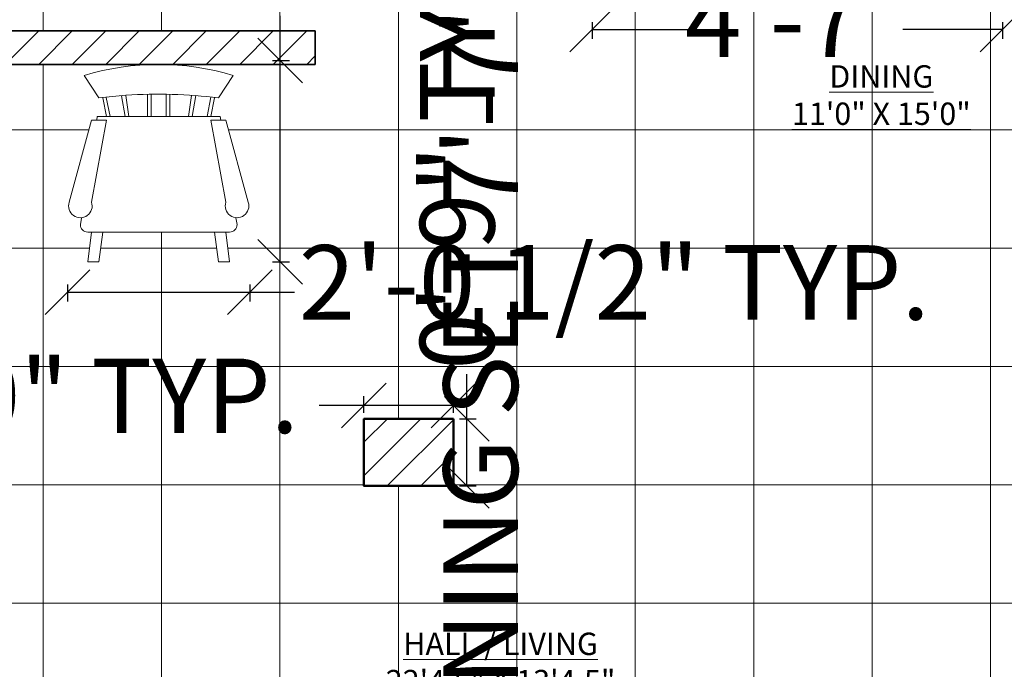
# Model space of a CAD drawing. Units: inches. Extents: x 2036 to 2670, y 319 to 920.
# Tile 5 of 15: x 2251 to 2383, y 579 to 666. Entities that reach past the tile are written whole.
import ezdxf

# ---------------------------------------------------------------- set-up
doc = ezdxf.new("R2010")
doc.units = ezdxf.units.IN
for name, color, linetype, lineweight in [('A-ANNO-DIMS', 2, 'Continuous', 18), ('A-AREA-IDEN', 7, 'Continuous', 18), ('A-COLS', 7, 'Continuous', 50), ('A-FLOR-PATT', 8, 'Continuous', 9), ('A-FURN', 8, 'Continuous', 18), ('A-WALL', 7, 'Continuous', 35)]:
    doc.layers.add(name, color=color, linetype=linetype, lineweight=lineweight)
doc.layers.add('A-COLS-PATT', color=240, linetype='Continuous', lineweight=13, true_color=0xed1f24)
doc.layers.add('A-WALL-PATT', color=52, linetype='Continuous', lineweight=13, true_color=0xc8c92d)
doc.styles.get("Standard").update_dxf_attribs({"font": 'arial.ttf'})
doc.dimstyles.new('ISO-25', dxfattribs={"dimtxt": 10, "dimasz": 6, "dimexe": 1.25, "dimexo": 0.625, "dimtad": 0, "dimdec": 1, "dimlunit": 3, "dimtxsty": 'Standard', "dimblk": 'OBLIQUE', "dimcen": 2.5, "dimclrd": 94, "dimclre": 94, "dimclrt": 1, "dimadec": 0, "dimazin": 0, "dimtfac": 1, "dimtdec": 1, "dimtmove": 0, "dimatfit": 3, "dimfxl": 1, "dimfxlon": 1, "dimarcsym": 0})

# ---------------------------------------------------------------- blocks, each defined once
blk = doc.blocks.new('Chair - Rocking')
for p, q in [((-8, -4.5), (-10, -1.5)), ((8, -4.5), (10, -1.5)), ((-7.5, -4.5), (-7, -7)), ((-6.5, -7), (-7.02225, -4.43)), ((-4.5, -7), (-4.96674, -4.19951)), ((-4, -7), (-4.40532, -4.16272)), ((-1.5, -4.05012), (-1.5, -7)), ((-1, -7), (-1, -4.05012)), ((1, -7), (1, -4.04655)), ((1.5, -4.05012), (1.5, -7)), ((4, -7), (4.40187, -4.18694)), ((4.5, -7), (4.96761, -4.19437)), ((6.5, -7), (7, -4.4057)), ((7.5, -4.5), (7, -7)), ((-9, -7.5), (-12, -18.49999)), ((-7, -7.5), (-9, -7.5)), ((-9, -18.49999), (-7, -7.5)), ((-8.23428, -6.99939), (-8.3093, -7.47958)), ((-8.23041, -7), (8.23915, -7)), ((7, -7.5), (9, -7.5)), ((9, -18.49999), (7, -7.5)), ((8.31071, -7.48854), (8.23449, -7.00073)), ((9, -7.5), (12, -18.49999)), ((-10.36644, -20.64523), (-10.5, -21.49999)), ((10.5, -21.49999), (10.3575, -20.58798)), ((-9, -22.49999), (-9.5, -26.49999)), ((0, -22.49999), (-9.5, -22.49999)), ((-8, -26.49999), (-7.5, -22.49999)), ((0, -22.49999), (9.5, -22.49999)), ((8, -26.49999), (7.5, -22.49999)), ((9, -22.49999), (9.5, -26.49999)), ((-9.5, -26.49999), (-8, -26.49999)), ((9.5, -26.49999), (8, -26.49999))]:
    blk.add_line(p, q)
for centre, radius, start, end in [((0, -34.08333), 34.08333, 72.93847, 107.0615), ((0, -68.25004), 64.25, 93.92211, 97.15267), ((0, -68.25004), 64.25, 82.84733, 93.92211), ((-10.5, -18.99999), 1.58114, 161.5651, 18.43495), ((10.5, -18.99999), 1.58114, 161.5651, 18.43495), ((-9.5, -21.49999), 1, 180, 270), ((9.5, -21.49999), 1, 270, 0)]:
    blk.add_arc(centre, radius, start, end)
blk = doc.blocks.new('COL-9x12')
blk.add_lwpolyline([(9, 0), (0, 0), (0, 12), (9, 12)], close=True)
blk = doc.blocks.new('_Oblique')
at = {"color": 0, "linetype": 'ByBlock', "lineweight": -2}
blk.add_line((-0.5, -0.5), (0.5, 0.5), dxfattribs=at)
blk = doc.blocks.new('*D21')
at = {"layer": 'A-ANNO-DIMS', "color": 94, "lineweight": -2, "transparency": 16777216}
for p, q in [((2297.27, 612.92), (2297.27, 615.17)), ((2309.27, 612.92), (2309.27, 615.17)), ((2297.27, 613.92), (2291.27, 613.92)), ((2309.27, 613.92), (2297.27, 613.92))]:
    blk.add_line(p, q, dxfattribs=at)
at = {"layer": 'Defpoints', "color": 0, "transparency": 16777216}
for p in [(2297.27, 613.92), (2297.27, 612.12), (2309.27, 612.12)]:
    blk.add_point(p, dxfattribs=at)
at = {"layer": 'A-ANNO-DIMS', "color": 94, "lineweight": -2, "transparency": 16777216, "xscale": 6, "yscale": 6, "zscale": 6}
for p, rotation in [((2297.27, 613.92), 179.9999999999962), ((2309.27, 613.92), 359.9999999999962)]:
    blk.add_blockref('_Oblique', p, dxfattribs=dict(at, rotation=rotation))
at = {"layer": 'A-ANNO-DIMS', "color": 1, "transparency": 16777216, "insert": (2228.01, 613.92), "char_height": 10, "attachment_point": 5}
blk.add_mtext('COLUMN 1\'-0" TYP.', dxfattribs=at)
blk = doc.blocks.new('*D22')
at = {"layer": 'A-ANNO-DIMS', "color": 94, "lineweight": -2, "transparency": 16777216}
for p, q in [((2311.07, 612.12), (2311.07, 618.12)), ((2310.07, 612.12), (2312.32, 612.12)), ((2311.07, 603.12), (2311.07, 612.12)), ((2310.07, 603.12), (2312.32, 603.12))]:
    blk.add_line(p, q, dxfattribs=at)
at = {"layer": 'Defpoints', "color": 0, "transparency": 16777216}
for p in [(2309.27, 612.12), (2311.07, 612.12), (2309.27, 603.12)]:
    blk.add_point(p, dxfattribs=at)
at = {"layer": 'A-ANNO-DIMS', "color": 94, "lineweight": -2, "transparency": 16777216, "xscale": 6, "yscale": 6, "zscale": 6}
for p, rotation in [((2311.07, 612.12), 90), ((2311.07, 603.12), 270)]:
    blk.add_blockref('_Oblique', p, dxfattribs=dict(at, rotation=rotation))
at = {"layer": 'A-ANNO-DIMS', "color": 1, "transparency": 16777216, "insert": (2311.07, 649.22), "char_height": 10, "attachment_point": 5, "rotation": 90}
blk.add_mtext('0\'-9" TYP.', dxfattribs=at)
blk = doc.blocks.new('*D23')
at = {"layer": 'A-ANNO-DIMS', "color": 94, "lineweight": -2, "transparency": 16777216}
for p, q in [((2286.03, 660.18), (2286.03, 666.18)), ((2285.03, 660.18), (2287.28, 660.18)), ((2286.03, 633.18), (2286.03, 660.18)), ((2285.03, 633.18), (2287.28, 633.18))]:
    blk.add_line(p, q, dxfattribs=at)
at = {"layer": 'Defpoints', "color": 0, "transparency": 16777216}
for p in [(2281.98, 660.18), (2286.03, 660.18), (2281.98, 633.18)]:
    blk.add_point(p, dxfattribs=at)
at = {"layer": 'A-ANNO-DIMS', "color": 94, "lineweight": -2, "transparency": 16777216, "xscale": 6, "yscale": 6, "zscale": 6}
for p, rotation in [((2286.03, 660.18), 90), ((2286.03, 633.18), 270)]:
    blk.add_blockref('_Oblique', p, dxfattribs=dict(at, rotation=rotation))
at = {"layer": 'A-ANNO-DIMS', "color": 1, "transparency": 16777216, "insert": (2286.03, 755.24), "char_height": 10, "attachment_point": 5, "rotation": 90}
blk.add_mtext('ROCKING CHAIR 2\'-3" TYP.', dxfattribs=at)
blk = doc.blocks.new('*D24')
at = {"layer": 'A-ANNO-DIMS', "color": 94, "lineweight": -2, "transparency": 16777216}
for p, q in [((2257.54, 630.13), (2257.54, 627.88)), ((2281.98, 630.13), (2281.98, 627.88)), ((2257.54, 629.13), (2281.98, 629.13)), ((2281.98, 629.13), (2287.98, 629.13))]:
    blk.add_line(p, q, dxfattribs=at)
at = {"layer": 'Defpoints', "color": 0, "transparency": 16777216}
for p in [(2257.54, 633.18), (2281.98, 633.18), (2281.98, 629.13)]:
    blk.add_point(p, dxfattribs=at)
at = {"layer": 'A-ANNO-DIMS', "color": 94, "lineweight": -2, "transparency": 16777216, "xscale": 6, "yscale": 6, "zscale": 6, "rotation": 180}
blk.add_blockref('_Oblique', (2257.54, 629.13), dxfattribs=at)
at = {"layer": 'A-ANNO-DIMS', "color": 94, "lineweight": -2, "transparency": 16777216, "xscale": 6, "yscale": 6, "zscale": 6}
blk.add_blockref('_Oblique', (2281.98, 629.13), dxfattribs=at)
at = {"layer": 'A-ANNO-DIMS', "color": 1, "transparency": 16777216, "insert": (2330.82, 629.13), "char_height": 10, "attachment_point": 5}
blk.add_mtext('2\'-0 1/2" TYP.', dxfattribs=at)
blk = doc.blocks.new('*D39')
at = {"layer": 'A-ANNO-DIMS', "color": 94, "lineweight": -2, "transparency": 16777216}
for p, q in [((2315.21, 769.01), (2312.96, 769.01)), ((2314.21, 769.01), (2314.21, 678.01)), ((2315.21, 678.01), (2312.96, 678.01)), ((2314.21, 678.01), (2314.21, 672.01))]:
    blk.add_line(p, q, dxfattribs=at)
at = {"layer": 'Defpoints', "color": 0, "transparency": 16777216}
for p in [(2327.86, 769.01), (2314.21, 678.01), (2327.86, 678.01)]:
    blk.add_point(p, dxfattribs=at)
at = {"layer": 'A-ANNO-DIMS', "color": 94, "lineweight": -2, "transparency": 16777216, "xscale": 6, "yscale": 6, "zscale": 6}
for p, rotation in [((2314.21, 769.01), 90), ((2314.21, 678.01), 270)]:
    blk.add_blockref('_Oblique', p, dxfattribs=dict(at, rotation=rotation))
at = {"layer": 'A-ANNO-DIMS', "color": 1, "transparency": 16777216, "insert": (2314.21, 616.43), "char_height": 10, "attachment_point": 5, "rotation": 90}
blk.add_mtext('DINING SET 7\'-7"', dxfattribs=at)
blk = doc.blocks.new('*D40')
at = {"layer": 'A-ANNO-DIMS', "color": 94, "lineweight": -2, "transparency": 16777216}
for p, q in [((2327.86, 665.36), (2327.86, 663.11)), ((2382.86, 665.36), (2382.86, 663.11)), ((2327.86, 664.36), (2341.24, 664.36)), ((2382.86, 664.36), (2369.48, 664.36))]:
    blk.add_line(p, q, dxfattribs=at)
at = {"layer": 'Defpoints', "color": 0, "transparency": 16777216}
for p in [(2327.86, 678.01), (2382.86, 678.01), (2382.86, 664.36)]:
    blk.add_point(p, dxfattribs=at)
at = {"layer": 'A-ANNO-DIMS', "color": 94, "lineweight": -2, "transparency": 16777216, "xscale": 6, "yscale": 6, "zscale": 6, "rotation": 180}
blk.add_blockref('_Oblique', (2327.86, 664.36), dxfattribs=at)
at = {"layer": 'A-ANNO-DIMS', "color": 94, "lineweight": -2, "transparency": 16777216, "xscale": 6, "yscale": 6, "zscale": 6}
blk.add_blockref('_Oblique', (2382.86, 664.36), dxfattribs=at)
at = {"layer": 'A-ANNO-DIMS', "color": 1, "transparency": 16777216, "insert": (2355.36, 664.36), "char_height": 10, "attachment_point": 5}
blk.add_mtext('4\'-7"', dxfattribs=at)
blk = doc.blocks.new('*D54')
at = {"layer": 'A-ANNO-DIMS', "color": 94, "lineweight": -2, "transparency": 16777216}
for p, q in [((2642.09, 545.51), (2642.09, 551.51)), ((2641.09, 545.51), (2643.34, 545.51)), ((2642.09, 513.19), (2642.09, 545.51)), ((2641.09, 513.19), (2643.34, 513.19))]:
    blk.add_line(p, q, dxfattribs=at)
at = {"layer": 'Defpoints', "color": 0, "transparency": 16777216}
for p in [(2158.74, 545.51), (2642.09, 545.51), (2158.74, 513.19)]:
    blk.add_point(p, dxfattribs=at)
at = {"layer": 'A-ANNO-DIMS', "color": 94, "lineweight": -2, "transparency": 16777216, "xscale": 6, "yscale": 6, "zscale": 6}
for p, rotation in [((2642.09, 545.51), 90), ((2642.09, 513.19), 270)]:
    blk.add_blockref('_Oblique', p, dxfattribs=dict(at, rotation=rotation))
at = {"layer": 'A-ANNO-DIMS', "color": 1, "transparency": 16777216, "insert": (2642.09, 577.16), "char_height": 10, "attachment_point": 5, "rotation": 90}
blk.add_mtext('2\'-8 1/2"', dxfattribs=at)
blk = doc.blocks.new('*D55')
at = {"layer": 'A-ANNO-DIMS', "color": 94, "lineweight": -2, "transparency": 16777216}
for p, q in [((2641.09, 582.53), (2643.34, 582.53)), ((2642.09, 582.53), (2642.09, 577.94)), ((2642.09, 545.51), (2642.09, 550.11)), ((2641.09, 545.51), (2643.34, 545.51))]:
    blk.add_line(p, q, dxfattribs=at)
at = {"layer": 'Defpoints', "color": 0, "transparency": 16777216}
for p in [(2158.74, 582.53), (2642.09, 582.53), (2158.74, 545.51)]:
    blk.add_point(p, dxfattribs=at)
at = {"layer": 'A-ANNO-DIMS', "color": 94, "lineweight": -2, "transparency": 16777216, "xscale": 6, "yscale": 6, "zscale": 6}
for p, rotation in [((2642.09, 582.53), 90), ((2642.09, 545.51), 270)]:
    blk.add_blockref('_Oblique', p, dxfattribs=dict(at, rotation=rotation))
at = {"layer": 'A-ANNO-DIMS', "color": 1, "transparency": 16777216, "insert": (2642.09, 564.02), "char_height": 10, "attachment_point": 5, "rotation": 90}
blk.add_mtext('3\'-1"', dxfattribs=at)
blk = doc.blocks.new('*D56')
at = {"layer": 'A-ANNO-DIMS', "color": 94, "lineweight": -2, "transparency": 16777216}
for p, q in [((2642.09, 599.85), (2642.09, 605.85)), ((2641.09, 599.85), (2643.34, 599.85)), ((2642.09, 582.53), (2642.09, 599.85)), ((2641.09, 582.53), (2643.34, 582.53))]:
    blk.add_line(p, q, dxfattribs=at)
at = {"layer": 'Defpoints', "color": 0, "transparency": 16777216}
for p in [(2158.74, 599.85), (2642.09, 599.85), (2158.74, 582.53)]:
    blk.add_point(p, dxfattribs=at)
at = {"layer": 'A-ANNO-DIMS', "color": 94, "lineweight": -2, "transparency": 16777216, "xscale": 6, "yscale": 6, "zscale": 6}
for p, rotation in [((2642.09, 599.85), 90), ((2642.09, 582.53), 270)]:
    blk.add_blockref('_Oblique', p, dxfattribs=dict(at, rotation=rotation))
at = {"layer": 'A-ANNO-DIMS', "color": 1, "transparency": 16777216, "insert": (2642.09, 630.95), "char_height": 10, "attachment_point": 5, "rotation": 90}
blk.add_mtext('1\'-5 1/2"', dxfattribs=at)
blk = doc.blocks.new('*D58')
at = {"layer": 'A-ANNO-DIMS', "color": 94, "lineweight": -2, "transparency": 16777216}
for p, q in [((2224.74, 436.33), (2224.74, 434.08)), ((2270.11, 436.33), (2270.11, 434.08)), ((2224.74, 435.33), (2270.11, 435.33)), ((2270.11, 435.33), (2276.11, 435.33))]:
    blk.add_line(p, q, dxfattribs=at)
at = {"layer": 'Defpoints', "color": 0, "transparency": 16777216}
for p in [(2224.74, 824.68), (2270.11, 824.68), (2270.11, 435.33)]:
    blk.add_point(p, dxfattribs=at)
at = {"layer": 'A-ANNO-DIMS', "color": 94, "lineweight": -2, "transparency": 16777216, "xscale": 6, "yscale": 6, "zscale": 6, "rotation": 180}
blk.add_blockref('_Oblique', (2224.74, 435.33), dxfattribs=at)
at = {"layer": 'A-ANNO-DIMS', "color": 94, "lineweight": -2, "transparency": 16777216, "xscale": 6, "yscale": 6, "zscale": 6}
blk.add_blockref('_Oblique', (2270.11, 435.33), dxfattribs=at)
at = {"layer": 'A-ANNO-DIMS', "color": 1, "transparency": 16777216, "insert": (2301.68, 435.33), "char_height": 10, "attachment_point": 5}
blk.add_mtext('3\'-9 1/2"', dxfattribs=at)
blk = doc.blocks.new('*D60')
at = {"layer": 'A-ANNO-DIMS', "color": 94, "lineweight": -2, "transparency": 16777216}
for p, q in [((2051.39, 582.41), (2051.39, 588.41)), ((2052.39, 582.41), (2050.14, 582.41)), ((2051.39, 545.09), (2051.39, 582.41)), ((2052.39, 545.09), (2050.14, 545.09))]:
    blk.add_line(p, q, dxfattribs=at)
at = {"layer": 'Defpoints', "color": 0, "transparency": 16777216}
for p in [(2051.39, 582.41), (2515.24, 582.41), (2515.24, 545.09)]:
    blk.add_point(p, dxfattribs=at)
at = {"layer": 'A-ANNO-DIMS', "color": 94, "lineweight": -2, "transparency": 16777216, "xscale": 6, "yscale": 6, "zscale": 6}
for p, rotation in [((2051.39, 582.41), 90), ((2051.39, 545.09), 270)]:
    blk.add_blockref('_Oblique', p, dxfattribs=dict(at, rotation=rotation))
at = {"layer": 'A-ANNO-DIMS', "color": 1, "transparency": 16777216, "insert": (2051.39, 613.98), "char_height": 10, "attachment_point": 5, "rotation": 90}
blk.add_mtext('3\'-1 1/2"', dxfattribs=at)

msp = doc.modelspace()

# ---------------------------------------------------------------- hatches: boundary and pattern name
at = {"layer": 'A-COLS-PATT'}
h = msp.add_hatch(dxfattribs=at)
h.set_pattern_fill('ANSI31', color=256)
h.paths.add_polyline_path([(2089.74, 875.68), (2080.74, 875.68), (2080.74, 863.68), (2089.74, 863.68)])
h.paths.add_polyline_path([(2089.74, 821.68), (2080.74, 821.68), (2080.74, 809.68), (2089.74, 809.68)])
h.paths.add_polyline_path([(2089.74, 624.2), (2080.74, 624.2), (2080.74, 612.2), (2089.74, 612.2)])
h.paths.add_polyline_path([(2158.74, 506.68), (2149.74, 506.68), (2149.74, 494.68), (2158.74, 494.68)])
h.paths.add_polyline_path([(2158.74, 617.33), (2149.74, 617.33), (2149.74, 605.33), (2158.74, 605.33)])
h.paths.add_polyline_path([(2158.74, 736.18), (2149.74, 736.18), (2149.74, 724.18), (2158.74, 724.18)])
h.paths.add_polyline_path([(2158.74, 852.81), (2149.74, 852.81), (2149.74, 843.81), (2158.74, 843.81)])
h.paths.add_polyline_path([(2161.74, 852.81), (2158.74, 852.81), (2158.74, 843.81), (2161.74, 843.81)])
h.paths.add_polyline_path([(2295.21, 857.66), (2290.74, 857.66), (2290.74, 848.68), (2295.21, 848.68)])
h.paths.add_polyline_path([(2290.74, 857.66), (2283.21, 857.66), (2283.21, 848.66), (2290.74, 848.66)])
h.paths.add_polyline_path([(2443.62, 857.68), (2431.62, 857.68), (2431.62, 848.68), (2443.62, 848.68)])
h.paths.add_polyline_path([(2561.81, 857.68), (2549.81, 857.68), (2549.81, 848.68), (2561.81, 848.68)])
h.paths.add_polyline_path([(2295.24, 737.65), (2290.74, 737.65), (2290.74, 728.68), (2295.24, 728.68)])
h.paths.add_polyline_path([(2309.27, 612.12), (2297.27, 612.12), (2297.27, 603.12), (2309.27, 603.12)])
h.paths.add_polyline_path([(2282.24, 503.68), (2270.24, 503.68), (2270.24, 494.68), (2282.24, 494.68)])
h.paths.add_polyline_path([(2431.74, 746.09), (2427.24, 746.09), (2427.24, 737.09), (2431.74, 737.09)])
h.paths.add_polyline_path([(2439.24, 746.09), (2431.74, 746.09), (2431.74, 737.09), (2439.24, 737.09)])
h.paths.add_polyline_path([(2596.59, 736.59), (2584.59, 736.59), (2584.59, 727.59), (2596.59, 727.59)])
h.paths.add_polyline_path([(2586.39, 623.71), (2574.39, 623.71), (2574.39, 619.18), (2586.39, 619.18)])
h.paths.add_polyline_path([(2586.39, 619.18), (2574.39, 619.18), (2574.39, 614.71), (2586.39, 614.71)])
h.paths.add_polyline_path([(2438.74, 623.68), (2431.24, 623.68), (2431.24, 619.18), (2438.74, 619.18)])
h.paths.add_polyline_path([(2438.74, 619.18), (2431.24, 619.18), (2431.24, 614.68), (2438.74, 614.68)])
h.paths.add_polyline_path([(2431.24, 623.68), (2426.74, 623.68), (2426.74, 614.68), (2431.24, 614.68), (2431.24, 619.18)])
h.paths.add_polyline_path([(2527.24, 503.68), (2515.24, 503.68), (2515.24, 494.68), (2527.24, 494.68)])
h.paths.add_polyline_path([(2590.31, 503.68), (2578.31, 503.68), (2578.31, 494.68), (2590.31, 494.68)])
at = {"layer": 'A-FLOR-PATT'}
h = msp.add_hatch(dxfattribs=at)
h.set_pattern_fill('ANSI31', color=256, scale=5, angle=135)
h.paths.add_polyline_path([(2290.74, 659.68), (2158.74, 659.68), (2158.74, 582.53), (2158.74, 545.51), (2158.74, 503.68), (2426.74, 503.68), (2426.74, 614.68), (2426.74, 623.68), (2426.74, 628.18), (2431.24, 628.18), (2431.24, 623.68), (2438.74, 623.68), (2438.74, 619.18), (2574.39, 619.18), (2574.39, 623.71), (2586.39, 623.71), (2586.39, 619.18), (2603.74, 619.18), (2603.74, 824.68), (2431.74, 824.68), (2431.74, 746.09), (2439.24, 746.09), (2439.24, 737.09), (2431.74, 737.09), (2431.74, 659.68), (2427.24, 659.68), (2427.24, 739.48), (2383.24, 739.48), (2383.24, 804.68), (2339.24, 804.68), (2339.24, 749.08), (2295.24, 749.08), (2295.24, 737.65), (2295.27, 737.65), (2295.27, 728.65), (2295.21, 728.65, -0.586418), (2272.74, 728.68), (2272.74, 824.68), (2270.11, 824.68), (2270.11, 829.18), (2290.74, 829.18), (2290.74, 848.66), (2283.21, 848.66), (2283.21, 857.66), (2289.74, 857.66), (2289.74, 874.68), (2158.74, 874.68), (2158.74, 852.81), (2161.74, 852.81), (2161.74, 843.81), (2158.74, 843.81), (2158.74, 829.18), (2224.74, 829.18), (2224.74, 800.68), (2182.74, 800.68), (2182.74, 733.41), (2158.74, 733.41), (2158.74, 728.68), (2235.24, 728.68), (2235.24, 714.81), (2230.74, 714.81), (2230.74, 724.18), (2158.74, 724.18), (2158.74, 664.18), (2230.74, 664.18), (2230.74, 678.81), (2235.24, 678.81), (2235.24, 664.18), (2290.74, 664.18)])
h.paths.add_polyline_path([(2309.27, 612.12), (2309.27, 603.12), (2297.27, 603.12), (2297.27, 612.12)], flags=16)
h.paths.add_polyline_path([(2280.12, 639.11), (2280.26, 638.18, -0.414214), (2279.26, 637.18), (2278.76, 637.18), (2279.26, 633.18), (2277.76, 633.18), (2277.26, 637.18), (2269.76, 637.18), (2262.26, 637.18), (2261.76, 633.18), (2260.26, 633.18), (2260.76, 637.18), (2260.26, 637.18, -0.414214), (2259.26, 638.18), (2259.41, 639.11, -0.541164), (2257.76, 641.18), (2260.76, 652.18), (2261.45, 652.18), (2261.53, 652.68), (2262.76, 652.68), (2262.25, 655.24, 0.001913), (2261.76, 655.18), (2259.76, 658.18, -0.15), (2279.76, 658.18), (2277.76, 655.18, 0.001913), (2277.27, 655.24), (2276.76, 652.68), (2278, 652.68), (2278.07, 652.18), (2278.76, 652.18), (2281.76, 641.18, -0.541163)], flags=16)
h.paths.add_polyline_path([(2245.98, 639.11), (2246.13, 638.18, -0.414214), (2245.13, 637.18), (2244.63, 637.18), (2245.13, 633.18), (2243.63, 633.18), (2243.13, 637.18), (2235.63, 637.18), (2228.13, 637.18), (2227.63, 633.18), (2226.13, 633.18), (2226.63, 637.18), (2226.13, 637.18, -0.414214), (2225.13, 638.18), (2225.27, 639.11, -0.541164), (2223.63, 641.18), (2226.63, 652.18), (2227.32, 652.18), (2227.39, 652.68), (2228.63, 652.68), (2228.12, 655.24, 0.001913), (2227.63, 655.18), (2225.63, 658.18, -0.15), (2245.63, 658.18), (2243.63, 655.18, 0.001913), (2243.14, 655.24), (2242.63, 652.68), (2243.86, 652.68), (2243.94, 652.18), (2244.63, 652.18), (2247.63, 641.18, -0.541163)], flags=16)
h.paths.add_polyline_path([(2351.59, 515.15, -0.151948), (2279.59, 515.15), (2279.59, 537.68), (2273.59, 537.68), (2273.59, 511.68, 0.190476), (2357.59, 511.68), (2357.59, 537.68), (2351.59, 537.68)])
h.paths.add_polyline_path([(2327.59, 536.13), (2327.59, 517.07), (2303.59, 517.07), (2303.59, 536.13)], flags=16)
h.paths.add_polyline_path([(2213.4, 639.11), (2213.55, 638.18, -0.414214), (2212.55, 637.18), (2212.05, 637.18), (2212.55, 633.18), (2211.05, 633.18), (2210.55, 637.18), (2203.05, 637.18), (2195.55, 637.18), (2195.05, 633.18), (2193.55, 633.18), (2194.05, 637.18), (2193.55, 637.18, -0.414214), (2192.55, 638.18), (2192.69, 639.11, -0.541164), (2191.05, 641.18), (2194.05, 652.18), (2194.73, 652.18), (2194.81, 652.68), (2196.05, 652.68), (2195.53, 655.24, 0.001913), (2195.05, 655.18), (2193.05, 658.18, -0.15), (2213.05, 658.18), (2211.05, 655.18, 0.001913), (2210.56, 655.24), (2210.05, 652.68), (2211.28, 652.68), (2211.36, 652.18), (2212.05, 652.18), (2215.05, 641.18, -0.541163)], flags=16)
h.paths.add_polyline_path([(2368.58, 538.02), (2370.52, 538.02), (2371.17, 532.84), (2380.89, 532.84), (2390.6, 532.84), (2391.25, 538.02), (2393.2, 538.02), (2392.55, 532.84), (2380.89, 532.84), (2368.58, 532.84, 0.414214), (2367.28, 531.54), (2367.47, 530.34, -0.483352), (2369.23, 527.65), (2371.82, 513.4), (2370.12, 513.4), (2370.22, 512.75), (2391.56, 512.75), (2391.66, 513.4), (2389.96, 513.4), (2392.55, 527.65, -1.387427), (2396.43, 527.65), (2392.55, 513.4), (2391.66, 513.4), (2391.56, 512.75), (2389.31, 512.75), (2390, 509.37, 0.003796), (2391.25, 509.51), (2393.84, 505.63, -0.15), (2367.93, 505.63), (2370.52, 509.51, 0.003901), (2371.81, 509.36), (2372.47, 512.75), (2370.22, 512.75), (2370.12, 513.4), (2369.23, 513.4), (2365.34, 527.65, -0.541163), (2367.47, 530.34), (2367.28, 531.54, -0.414214), (2368.58, 532.84), (2369.23, 532.84)])
h.paths.add_polyline_path([(2266.74, 538.02), (2266.09, 532.84), (2254.43, 532.84), (2242.12, 532.84, 0.414214), (2240.83, 531.54), (2241.01, 530.34, -0.483352), (2242.77, 527.65), (2245.36, 513.4), (2243.66, 513.4), (2243.76, 512.75), (2265.1, 512.75), (2265.2, 513.4), (2263.5, 513.4), (2266.09, 527.65, -1.387427), (2269.98, 527.65), (2266.09, 513.4), (2265.2, 513.4), (2265.1, 512.75), (2262.85, 512.75), (2263.54, 509.37, 0.003796), (2264.79, 509.51), (2267.39, 505.63, -0.15), (2241.47, 505.63), (2244.07, 509.51, 0.003901), (2245.36, 509.36), (2246.01, 512.75), (2243.76, 512.75), (2243.66, 513.4), (2242.77, 513.4), (2238.88, 527.65, -0.541163), (2241.01, 530.34), (2240.83, 531.54, -0.414214), (2242.12, 532.84), (2242.77, 532.84), (2242.12, 538.02), (2244.07, 538.02), (2244.71, 532.84), (2254.43, 532.84), (2264.15, 532.84), (2264.79, 538.02)])
h.paths.add_polyline_path([(2185.24, 620.36), (2185.24, 618.86), (2181.24, 618.36), (2181.24, 610.86), (2181.24, 603.36), (2185.24, 602.86), (2185.24, 601.36), (2181.24, 601.86), (2181.24, 601.36, -0.414214), (2180.24, 600.36), (2179.31, 600.5, -0.541164), (2177.24, 598.86), (2166.24, 601.86), (2166.24, 602.54), (2165.74, 602.62), (2165.74, 603.86), (2163.18, 603.34, 0.001913), (2163.24, 602.86), (2160.24, 600.86, -0.15), (2160.24, 620.86), (2163.24, 618.86, 0.001913), (2163.18, 618.37), (2165.74, 617.86), (2165.74, 619.09), (2166.24, 619.17), (2166.24, 619.86), (2177.24, 622.86, -0.541163), (2179.31, 621.21), (2180.24, 621.36, -0.414214), (2181.24, 620.36), (2181.24, 619.86)])
h.paths.add_polyline_path([(2470.92, 676.01), (2470.92, 806.13), (2568.52, 806.13), (2568.52, 676.01)], flags=16)
h.paths.add_polyline_path([(2177.74, 677.49), (2161.9, 677.49), (2161.9, 705.85), (2177.74, 705.85)], flags=16)
h.paths.add_polyline_path([(2176.74, 678.49), (2162.9, 678.49), (2162.9, 704.85), (2176.74, 704.85)], flags=0)
h.paths.add_polyline_path([(2175.01, 686.48), (2172.93, 686.48), (2172.93, 690.63), (2170.86, 690.63), (2170.86, 686.48), (2164.63, 686.48), (2164.63, 688.56), (2166.71, 688.56), (2168.78, 688.56), (2168.78, 690.63), (2164.63, 690.63), (2164.63, 696.85), (2166.71, 696.85), (2166.71, 692.71), (2168.78, 692.71), (2168.78, 696.85), (2175.01, 696.85), (2175.01, 694.78), (2170.86, 694.78), (2170.86, 692.71), (2175.01, 692.71)], flags=0)
h.paths.add_polyline_path([(2543.79, 782.71), (2483.94, 782.71), (2483.94, 804.18), (2517.77, 804.18), (2517.77, 782.71), (2521.67, 782.71), (2521.67, 804.18), (2555.5, 804.18), (2555.5, 779.45), (2547.05, 779.45), (2568.52, 757.98), (2543.79, 757.98)], flags=0)
h.paths.add_polyline_path([(2584.59, 727.59), (2584.59, 736.59), (2596.59, 736.59), (2596.59, 727.59)], flags=16)
h.paths.add_polyline_path([(2520.45, 647.03), (2553.79, 647.03), (2553.79, 658.23), (2520.45, 658.23)], flags=24)
h.paths.add_polyline_path([(2299.53, 573.74), (2331.71, 573.74), (2331.71, 584.94), (2299.53, 584.94)], flags=24)
h.paths.add_polyline_path([(2191.59, 685.19), (2212.12, 685.19), (2212.12, 696.38), (2191.59, 696.38)], flags=24)
h.paths.add_polyline_path([(2353.9, 649.86), (2379.08, 649.86), (2379.08, 661.06), (2353.9, 661.06)], flags=24)
h.paths.add_polyline_path([(2214.61, 763.31), (2237.46, 763.31), (2237.46, 779.56), (2214.61, 779.56)], flags=24)
h.paths.add_polyline_path([(2225.09, 819.31), (2269.29, 819.31), (2269.29, 844.04), (2225.09, 844.04)], flags=24)
h.paths.add_polyline_path([(2204.06, 845.04), (2226.92, 845.04), (2226.92, 856.24), (2204.06, 856.24)], flags=24)
h = msp.add_hatch(dxfattribs=at)
h.set_pattern_fill('ANSI31', color=256, scale=5, angle=45)
h.paths.add_polyline_path([(2290.74, 659.68), (2158.74, 659.68), (2158.74, 582.53), (2158.74, 545.51), (2158.74, 503.68), (2426.74, 503.68), (2426.74, 614.68), (2426.74, 623.68), (2426.74, 628.18), (2431.24, 628.18), (2431.24, 623.68), (2438.74, 623.68), (2438.74, 619.18), (2574.39, 619.18), (2574.39, 623.71), (2586.39, 623.71), (2586.39, 619.18), (2603.74, 619.18), (2603.74, 824.68), (2431.74, 824.68), (2431.74, 746.09), (2439.24, 746.09), (2439.24, 737.09), (2431.74, 737.09), (2431.74, 659.68), (2427.24, 659.68), (2427.24, 739.48), (2383.24, 739.48), (2383.24, 804.68), (2339.24, 804.68), (2339.24, 749.08), (2295.24, 749.08), (2295.24, 737.65), (2295.27, 737.65), (2295.27, 728.65), (2295.21, 728.65, -0.586418), (2272.74, 728.68), (2272.74, 824.68), (2270.11, 824.68), (2270.11, 829.18), (2290.74, 829.18), (2290.74, 848.66), (2283.21, 848.66), (2283.21, 857.66), (2289.74, 857.66), (2289.74, 874.68), (2158.74, 874.68), (2158.74, 852.81), (2161.74, 852.81), (2161.74, 843.81), (2158.74, 843.81), (2158.74, 829.18), (2224.74, 829.18), (2224.74, 800.68), (2182.74, 800.68), (2182.74, 733.41), (2158.74, 733.41), (2158.74, 728.68), (2235.24, 728.68), (2235.24, 714.81), (2230.74, 714.81), (2230.74, 724.18), (2158.74, 724.18), (2158.74, 664.18), (2230.74, 664.18), (2230.74, 678.81), (2235.24, 678.81), (2235.24, 664.18), (2290.74, 664.18)])
h.paths.add_polyline_path([(2309.27, 612.12), (2309.27, 603.12), (2297.27, 603.12), (2297.27, 612.12)], flags=16)
h.paths.add_polyline_path([(2280.12, 639.11), (2280.26, 638.18, -0.414214), (2279.26, 637.18), (2278.76, 637.18), (2279.26, 633.18), (2277.76, 633.18), (2277.26, 637.18), (2269.76, 637.18), (2262.26, 637.18), (2261.76, 633.18), (2260.26, 633.18), (2260.76, 637.18), (2260.26, 637.18, -0.414214), (2259.26, 638.18), (2259.41, 639.11, -0.541164), (2257.76, 641.18), (2260.76, 652.18), (2261.45, 652.18), (2261.53, 652.68), (2262.76, 652.68), (2262.25, 655.24, 0.001913), (2261.76, 655.18), (2259.76, 658.18, -0.15), (2279.76, 658.18), (2277.76, 655.18, 0.001913), (2277.27, 655.24), (2276.76, 652.68), (2278, 652.68), (2278.07, 652.18), (2278.76, 652.18), (2281.76, 641.18, -0.541163)], flags=16)
h.paths.add_polyline_path([(2245.98, 639.11), (2246.13, 638.18, -0.414214), (2245.13, 637.18), (2244.63, 637.18), (2245.13, 633.18), (2243.63, 633.18), (2243.13, 637.18), (2235.63, 637.18), (2228.13, 637.18), (2227.63, 633.18), (2226.13, 633.18), (2226.63, 637.18), (2226.13, 637.18, -0.414214), (2225.13, 638.18), (2225.27, 639.11, -0.541164), (2223.63, 641.18), (2226.63, 652.18), (2227.32, 652.18), (2227.39, 652.68), (2228.63, 652.68), (2228.12, 655.24, 0.001913), (2227.63, 655.18), (2225.63, 658.18, -0.15), (2245.63, 658.18), (2243.63, 655.18, 0.001913), (2243.14, 655.24), (2242.63, 652.68), (2243.86, 652.68), (2243.94, 652.18), (2244.63, 652.18), (2247.63, 641.18, -0.541163)], flags=16)
h.paths.add_polyline_path([(2351.59, 537.68), (2351.59, 515.15, -0.151948), (2279.59, 515.15), (2279.59, 537.68), (2273.59, 537.68), (2273.59, 511.68, 0.190476), (2357.59, 511.68), (2357.59, 537.68)])
h.paths.add_polyline_path([(2368.58, 538.02), (2370.52, 538.02), (2371.17, 532.84), (2380.89, 532.84), (2390.6, 532.84), (2391.25, 538.02), (2393.2, 538.02), (2392.55, 532.84), (2380.89, 532.84), (2368.58, 532.84, 0.414214), (2367.28, 531.54), (2367.47, 530.34, -0.483352), (2369.23, 527.65), (2371.82, 513.4), (2370.12, 513.4), (2370.22, 512.75), (2391.56, 512.75), (2391.66, 513.4), (2389.96, 513.4), (2392.55, 527.65, -1.387427), (2396.43, 527.65), (2392.55, 513.4), (2391.66, 513.4), (2391.56, 512.75), (2389.31, 512.75), (2390, 509.37, 0.003796), (2391.25, 509.51), (2393.84, 505.63, -0.15), (2367.93, 505.63), (2370.52, 509.51, 0.003901), (2371.81, 509.36), (2372.47, 512.75), (2370.22, 512.75), (2370.12, 513.4), (2369.23, 513.4), (2365.34, 527.65, -0.541163), (2367.47, 530.34), (2367.28, 531.54, -0.414214), (2368.58, 532.84), (2369.23, 532.84)])
h.paths.add_polyline_path([(2327.59, 536.13), (2327.59, 517.07), (2303.59, 517.07), (2303.59, 536.13)], flags=16)
h.paths.add_polyline_path([(2470.92, 676.01), (2470.92, 806.13), (2568.52, 806.13), (2568.52, 676.01)], flags=16)
h.paths.add_polyline_path([(2266.74, 538.02), (2266.09, 532.84), (2254.43, 532.84), (2242.12, 532.84, 0.414214), (2240.83, 531.54), (2241.01, 530.34, -0.483352), (2242.77, 527.65), (2245.36, 513.4), (2243.66, 513.4), (2243.76, 512.75), (2265.1, 512.75), (2265.2, 513.4), (2263.5, 513.4), (2266.09, 527.65, -1.387427), (2269.98, 527.65), (2266.09, 513.4), (2265.2, 513.4), (2265.1, 512.75), (2262.85, 512.75), (2263.54, 509.37, 0.003796), (2264.79, 509.51), (2267.39, 505.63, -0.15), (2241.47, 505.63), (2244.07, 509.51, 0.003901), (2245.36, 509.36), (2246.01, 512.75), (2243.76, 512.75), (2243.66, 513.4), (2242.77, 513.4), (2238.88, 527.65, -0.541163), (2241.01, 530.34), (2240.83, 531.54, -0.414214), (2242.12, 532.84), (2242.77, 532.84), (2242.12, 538.02), (2244.07, 538.02), (2244.71, 532.84), (2254.43, 532.84), (2264.15, 532.84), (2264.79, 538.02)])
h.paths.add_polyline_path([(2213.4, 639.11), (2213.55, 638.18, -0.414214), (2212.55, 637.18), (2212.05, 637.18), (2212.55, 633.18), (2211.05, 633.18), (2210.55, 637.18), (2203.05, 637.18), (2195.55, 637.18), (2195.05, 633.18), (2193.55, 633.18), (2194.05, 637.18), (2193.55, 637.18, -0.414214), (2192.55, 638.18), (2192.69, 639.11, -0.541164), (2191.05, 641.18), (2194.05, 652.18), (2194.73, 652.18), (2194.81, 652.68), (2196.05, 652.68), (2195.53, 655.24, 0.001913), (2195.05, 655.18), (2193.05, 658.18, -0.15), (2213.05, 658.18), (2211.05, 655.18, 0.001913), (2210.56, 655.24), (2210.05, 652.68), (2211.28, 652.68), (2211.36, 652.18), (2212.05, 652.18), (2215.05, 641.18, -0.541163)], flags=16)
h.paths.add_polyline_path([(2185.24, 620.36), (2185.24, 618.86), (2181.24, 618.36), (2181.24, 610.86), (2181.24, 603.36), (2185.24, 602.86), (2185.24, 601.36), (2181.24, 601.86), (2181.24, 601.36, -0.414214), (2180.24, 600.36), (2179.31, 600.5, -0.541164), (2177.24, 598.86), (2166.24, 601.86), (2166.24, 602.54), (2165.74, 602.62), (2165.74, 603.86), (2163.18, 603.34, 0.001913), (2163.24, 602.86), (2160.24, 600.86, -0.15), (2160.24, 620.86), (2163.24, 618.86, 0.001913), (2163.18, 618.37), (2165.74, 617.86), (2165.74, 619.09), (2166.24, 619.17), (2166.24, 619.86), (2177.24, 622.86, -0.541163), (2179.31, 621.21), (2180.24, 621.36, -0.414214), (2181.24, 620.36), (2181.24, 619.86)])
h.paths.add_polyline_path([(2177.74, 677.49), (2161.9, 677.49), (2161.9, 705.85), (2177.74, 705.85)], flags=16)
h.paths.add_polyline_path([(2176.74, 678.49), (2162.9, 678.49), (2162.9, 704.85), (2176.74, 704.85)], flags=0)
h.paths.add_polyline_path([(2175.01, 686.48), (2172.93, 686.48), (2172.93, 690.63), (2170.86, 690.63), (2170.86, 686.48), (2164.63, 686.48), (2164.63, 688.56), (2166.71, 688.56), (2168.78, 688.56), (2168.78, 690.63), (2164.63, 690.63), (2164.63, 696.85), (2166.71, 696.85), (2166.71, 692.71), (2168.78, 692.71), (2168.78, 696.85), (2175.01, 696.85), (2175.01, 694.78), (2170.86, 694.78), (2170.86, 692.71), (2175.01, 692.71)], flags=0)
h.paths.add_polyline_path([(2543.79, 782.71), (2483.94, 782.71), (2483.94, 804.18), (2517.77, 804.18), (2517.77, 782.71), (2521.67, 782.71), (2521.67, 804.18), (2555.5, 804.18), (2555.5, 779.45), (2547.05, 779.45), (2568.52, 757.98), (2543.79, 757.98)], flags=0)
h.paths.add_polyline_path([(2584.59, 727.59), (2584.59, 736.59), (2596.59, 736.59), (2596.59, 727.59)], flags=16)
h.paths.add_polyline_path([(2520.45, 647.03), (2553.79, 647.03), (2553.79, 658.23), (2520.45, 658.23)], flags=24)
h.paths.add_polyline_path([(2299.53, 573.74), (2331.71, 573.74), (2331.71, 584.94), (2299.53, 584.94)], flags=24)
h.paths.add_polyline_path([(2191.59, 685.19), (2212.12, 685.19), (2212.12, 696.38), (2191.59, 696.38)], flags=24)
h.paths.add_polyline_path([(2353.9, 649.86), (2379.08, 649.86), (2379.08, 661.06), (2353.9, 661.06)], flags=24)
h.paths.add_polyline_path([(2214.61, 763.31), (2237.46, 763.31), (2237.46, 779.56), (2214.61, 779.56)], flags=24)
h.paths.add_polyline_path([(2225.09, 819.31), (2269.29, 819.31), (2269.29, 844.04), (2225.09, 844.04)], flags=24)
h.paths.add_polyline_path([(2204.06, 845.04), (2226.92, 845.04), (2226.92, 856.24), (2204.06, 856.24)], flags=24)
h = msp.add_hatch(dxfattribs=at)
h.set_pattern_fill('ANSI31', color=256, scale=3, angle=135)
h.paths.add_polyline_path([(2149.74, 582.53), (2149.74, 707.68), (2120.74, 707.68), (2120.74, 599.68, -1), (2118.74, 599.68), (2085.24, 599.68), (2085.24, 506.68), (2089.74, 506.68), (2089.74, 494.68), (2085.24, 494.68), (2085.24, 469.18), (2608.24, 469.18), (2608.24, 494.68), (2149.74, 494.68), (2149.74, 506.68), (2149.74, 545.51)])
h.paths.add_polyline_path([(2143.58, 686.71), (2149.03, 686.71), (2149.03, 692.89), (2143.58, 692.89)], flags=24)
h.paths.add_polyline_path([(2125.99, 700.31), (2133.31, 700.31), (2133.31, 706.49), (2125.99, 706.49)], flags=24)
at = {"layer": 'A-WALL-PATT'}
h = msp.add_hatch(dxfattribs=at)
h.set_pattern_fill('ANSI31', color=256)
h.paths.add_polyline_path([(2089.74, 863.68), (2080.74, 863.68), (2080.74, 821.68), (2089.74, 821.68)])
h.paths.add_polyline_path([(2089.74, 809.68), (2080.74, 809.68), (2080.74, 624.2), (2089.74, 624.2), (2089.74, 707.68), (2089.74, 767.68)])
h.paths.add_polyline_path([(2149.74, 818.68), (2089.74, 818.68), (2089.74, 809.68), (2149.74, 809.68)])
h.paths.add_polyline_path([(2158.74, 875.68), (2089.74, 875.68), (2089.74, 866.68), (2149.74, 866.68), (2149.74, 852.81), (2158.74, 852.81)])
h.paths.add_polyline_path([(2158.74, 843.81), (2149.74, 843.81), (2149.74, 736.18), (2158.74, 736.18), (2158.74, 824.68)])
h.paths.add_polyline_path([(2181.31, 829.18), (2158.74, 829.18), (2158.74, 824.68), (2181.31, 824.68)])
h.paths.add_polyline_path([(2224.74, 829.18), (2212.72, 829.18), (2212.72, 824.68), (2224.74, 824.68)])
h.paths.add_polyline_path([(2177.02, 503.68), (2158.74, 503.68), (2158.74, 494.68), (2177.02, 494.68)])
h.paths.add_polyline_path([(2158.74, 664.18), (2158.74, 680.02), (2149.74, 680.02), (2149.74, 617.33), (2158.74, 617.33)])
h.paths.add_polyline_path([(2158.74, 724.18), (2149.74, 724.18), (2149.74, 704.02), (2158.74, 704.02)])
h.paths.add_polyline_path([(2235.24, 728.68), (2158.74, 728.68), (2158.74, 724.18), (2230.74, 724.18), (2230.74, 714.81), (2235.24, 714.81)])
h.paths.add_polyline_path([(2290.74, 664.18), (2235.24, 664.18), (2235.24, 678.81), (2230.74, 678.81), (2230.74, 664.18), (2158.74, 664.18), (2158.74, 659.68), (2290.74, 659.68)])
h.paths.add_polyline_path([(2270.24, 503.68), (2227.17, 503.68), (2227.17, 494.68), (2270.24, 494.68)])
h.paths.add_polyline_path([(2515.24, 503.68), (2380.89, 503.68), (2380.89, 494.68), (2515.24, 494.68)])
h.paths.add_polyline_path([(2292.21, 503.68), (2282.24, 503.68), (2282.24, 494.68), (2292.21, 494.68)])
h.paths.add_polyline_path([(2578.31, 503.68), (2527.24, 503.68), (2527.24, 494.68), (2578.31, 494.68)])
h.paths.add_polyline_path([(2603.74, 503.68), (2590.31, 503.68), (2590.31, 494.68), (2603.74, 494.68)])
h.paths.add_polyline_path([(2612.74, 503.68), (2603.74, 503.68), (2603.74, 494.68), (2612.74, 494.68)])
h.paths.add_polyline_path([(2549.81, 857.68), (2443.62, 857.68), (2443.62, 848.68), (2549.81, 848.68)])
h.paths.add_polyline_path([(2295.24, 848.66), (2290.74, 848.66), (2290.74, 829.18), (2270.11, 829.18), (2270.11, 824.68), (2290.74, 824.68), (2290.74, 737.65), (2295.24, 737.65)])
h.paths.add_polyline_path([(2431.74, 737.09), (2427.24, 737.09), (2427.24, 659.68), (2431.74, 659.68)])
h.paths.add_polyline_path([(2431.74, 848.68), (2427.24, 848.68), (2427.24, 746.09), (2431.74, 746.09)])
h.paths.add_polyline_path([(2574.39, 619.18), (2495.46, 619.18), (2495.46, 614.68), (2574.39, 614.68)])
h.paths.add_polyline_path([(2461.84, 619.18), (2438.74, 619.18), (2438.74, 614.68), (2461.84, 614.68)])
h.paths.add_polyline_path([(2603.74, 619.18), (2586.39, 619.18), (2586.39, 614.68), (2603.74, 614.68)], flags=17)

# ---------------------------------------------------------------- linework, layer by layer
at = {"layer": 'A-WALL'}
for p, q in [((2235.24, 664.18), (2290.74, 664.18)), ((2290.74, 664.18), (2290.74, 659.68)), ((2158.74, 659.68), (2290.74, 659.68))]:
    msp.add_line(p, q, dxfattribs=at)

# ---------------------------------------------------------------- block references
at = {"layer": 'A-COLS', "rotation": 89.99999999999625}
msp.add_blockref('COL-9x12', (2309.27, 603.12), dxfattribs=at)
at = {"layer": 'A-FURN'}
msp.add_blockref('Chair - Rocking', (2269.76, 659.68), dxfattribs=at)

# ---------------------------------------------------------------- texts
at = {"layer": 'A-AREA-IDEN', "char_height": 3, "attachment_point": 1}
for s, width, insert in [('\\pxqc;{\\LDINING\\P11\'0" X 15\'0"}', 24.0713, (2354.58, 659.56)), ('\\pxqc;{\\LHALL / LIVING\\P22\'4.5" X 13\'4.5"}', 36.9116, (2297.13, 583.44))]:
    msp.add_mtext_dynamic_manual_height_columns(s, width=width, gutter_width=12.5, heights=[0], dxfattribs=dict(at, insert=insert))

# ---------------------------------------------------------------- dimensions: what is measured, and where the dimension line sits
at = {"layer": 'A-ANNO-DIMS'}
for base, p1, p2, angle, text, picture, middle in [((2286.03, 660.18), (2281.98, 633.18), (2281.98, 660.18), 90, 'ROCKING CHAIR <> TYP.', '*D23', (2286.03, 755.24)), ((2314.21, 678.01), (2327.86, 769.01), (2327.86, 678.01), 270, 'DINING SET <>', '*D39', (2314.21, 616.43)), ((2311.07, 612.12), (2309.27, 603.12), (2309.27, 612.12), 90, '<> TYP.', '*D22', (2311.07, 649.22)), ((2297.27, 613.92), (2309.27, 612.12), (2297.27, 612.12), 180, 'COLUMN <> TYP.', '*D21', (2228.01, 613.92))]:
    dim = msp.add_linear_dim(base=base, p1=p1, p2=p2, angle=angle, text=text, dimstyle='ISO-25', override={"dimdec": 1, "dimlfac": 1, "dimrnd": 0, "dimzin": 1, "dimdsep": 46, "dimlunit": 4, "dimfrac": 2}, dxfattribs=at)
    dim.commit()
    dim.dimension.update_dxf_attribs({"geometry": picture, "text_midpoint": middle})
for base, p1, p2, picture, middle in [((2270.11, 435.33), (2224.74, 824.68), (2270.11, 824.68), '*D58', (2301.68, 435.33)), ((2382.86, 664.36), (2327.86, 678.01), (2382.86, 678.01), '*D40', (2355.36, 664.36))]:
    dim = msp.add_linear_dim(base=base, p1=p1, p2=p2, dimstyle='ISO-25', override={"dimdec": 1, "dimlfac": 1, "dimrnd": 0, "dimzin": 1, "dimdsep": 46, "dimlunit": 4, "dimfrac": 2}, dxfattribs=at)
    dim.commit()
    dim.dimension.update_dxf_attribs({"geometry": picture, "text_midpoint": middle})
for base, p1, p2, picture, middle in [((2642.09, 599.85), (2158.74, 582.53), (2158.74, 599.85), '*D56', (2642.09, 630.95)), ((2051.39, 582.41), (2515.24, 545.09), (2515.24, 582.41), '*D60', (2051.39, 613.98)), ((2642.09, 545.51), (2158.74, 513.19), (2158.74, 545.51), '*D54', (2642.09, 577.16)), ((2642.09, 582.53), (2158.74, 545.51), (2158.74, 582.53), '*D55', (2642.09, 564.02))]:
    dim = msp.add_linear_dim(base=base, p1=p1, p2=p2, angle=90, dimstyle='ISO-25', override={"dimdec": 1, "dimlfac": 1, "dimrnd": 0, "dimzin": 1, "dimdsep": 46, "dimlunit": 4, "dimfrac": 2}, dxfattribs=at)
    dim.commit()
    dim.dimension.update_dxf_attribs({"geometry": picture, "text_midpoint": middle})
dim = msp.add_linear_dim(base=(2281.98, 629.13), p1=(2257.54, 633.18), p2=(2281.98, 633.18), text='<> TYP.', dimstyle='ISO-25', override={"dimdec": 1, "dimlfac": 1, "dimrnd": 0, "dimzin": 1, "dimdsep": 46, "dimlunit": 4, "dimfrac": 2}, dxfattribs=at)
dim.commit()
dim.dimension.update_dxf_attribs({"geometry": '*D24', "text_midpoint": (2330.82, 629.13)})

doc.saveas('drawing.dxf')
